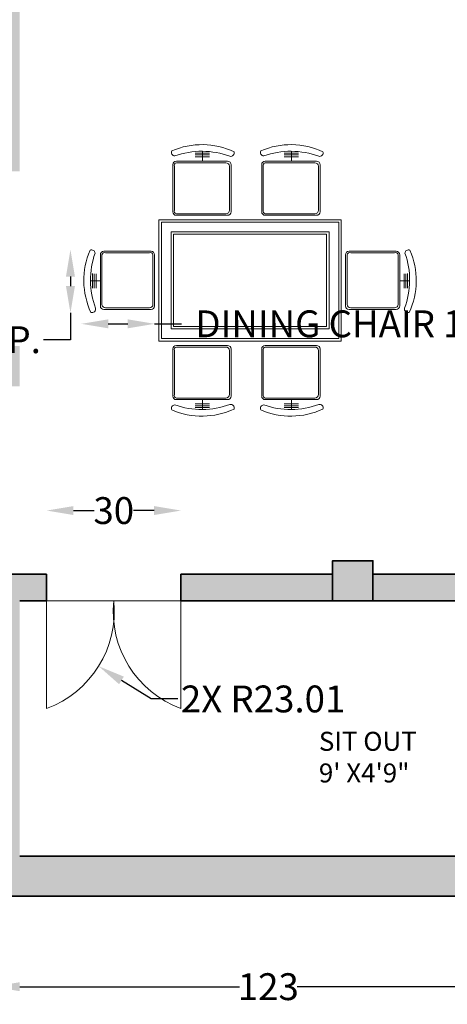
# Model space of a CAD drawing. Units: inches. Extents: x 1994 to 3075, y 3517 to 3950.
# Tile 53 of 58: x 2816 to 2912, y 3517 to 3737. Entities that reach past the tile are written whole.
import ezdxf

# ---------------------------------------------------------------- set-up
doc = ezdxf.new("R2010")
doc.units = ezdxf.units.IN
for name, color, linetype, lineweight in [('A-ANNO-DIMS', 2, 'Continuous', 18), ('A-AREA-IDEN', 7, 'Continuous', 18), ('A-COLS', 7, 'Continuous', 35), ('A-COLS-PATT', 6, 'Continuous', 13), ('A-DOOR', 3, 'Continuous', 18), ('A-FURN', 8, 'Continuous', 18), ('A-WALL', 7, 'Continuous', 35), ('A-WALL-PATT', 252, 'Continuous', 13)]:
    doc.layers.add(name, color=color, linetype=linetype, lineweight=lineweight)
doc.styles.get("Standard").update_dxf_attribs({"font": 'arial.ttf'})
doc.dimstyles.get("Standard").update_dxf_attribs({"dimtxt": 6, "dimasz": 6, "dimexe": 0.18, "dimexo": 0.0625, "dimgap": 0.09, "dimtad": 0, "dimtih": 1, "dimtoh": 1, "dimdec": 4, "dimzin": 0, "dimdsep": 46, "dimlunit": 4, "dimtxsty": 'Standard', "dimcen": 0.09, "dimse1": 1, "dimse2": 1, "dimadec": 0, "dimazin": 0, "dimtfac": 1, "dimtdec": 4, "dimtofl": 0, "dimtmove": 0, "dimatfit": 3, "dimfxl": 1, "dimtolj": 1, "dimtzin": 0, "dimarcsym": 0})

# ---------------------------------------------------------------- blocks, each defined once
blk = doc.blocks.new('CHAIR-DINING')
for p, q in [((12.53, 15.8), (1.1, 15.8)), ((12.17, 15.44), (1.1, 15.44)), ((0.3, 15), (0.3, 4.49)), ((0.66, 14.64), (0.66, 4.85)), ((12.97, 4.85), (12.97, 14.64)), ((13.33, 4.49), (13.33, 15)), ((1.1, 4.05), (12.17, 4.05)), ((1.1, 3.69), (12.53, 3.69)), ((5.32, 2.73), (8.52, 2.73)), ((5.32, 2.3), (8.52, 2.3)), ((6.92, 3.69), (6.92, 1.56)), ((5.29, 1.93), (8.52, 1.93))]:
    blk.add_line(p, q)
for centre, radius, start, end in [((1.1, 15), 0.8, 90, 180), ((1.17, 14.88), 0.564, 96.7142, 205.1766), ((12.17, 14.64), 0.8, 0, 90), ((12.53, 15), 0.8, 0, 90), ((1.1, 4.49), 0.8, 180, 270), ((1.17, 4.61), 0.564, 154.8234, 263.2858), ((12.17, 4.85), 0.8, 270, 0), ((12.53, 4.49), 0.8, 270, 0), ((0.77, 1.75), 0.766, 91.9354, 207.5327), ((6.77, 19.53), 18.05, 250.4914, 290.3763), ((13.22, 1.83), 0.8, 342.1953, 102.3742), ((6.83, 16.94), 16.94, 246.5531, 294.9844)]:
    blk.add_arc(centre, radius, start, end)
blk = doc.blocks.new('*D15')
at = {"layer": 'A-ANNO-DIMS', "color": 0, "lineweight": -2, "transparency": 16777216}
for p, q in [((2835.85, 3669.06), (2840.19, 3669.06)), ((2846.19, 3669.06), (2852.19, 3669.06))]:
    blk.add_line(p, q, dxfattribs=at)
at = {"layer": 'A-ANNO-DIMS', "color": 0, "transparency": 16777216}
for points in [[(2835.85, 3670.06), (2835.85, 3668.06), (2829.85, 3669.06)], [(2840.19, 3670.06), (2840.19, 3668.06), (2846.19, 3669.06)]]:
    blk.add_solid(points, dxfattribs=at)
at = {"layer": 'Defpoints', "color": 0, "transparency": 16777216}
for p in [(2829.85, 3671.51), (2846.19, 3671.51), (2846.19, 3669.06)]:
    blk.add_point(p, dxfattribs=at)
at = {"layer": 'A-ANNO-DIMS', "color": 0, "transparency": 16777216, "insert": (2896.77, 3669.06), "char_height": 6, "attachment_point": 5}
blk.add_mtext('\\A1;DINING CHAIR 16 TYP.', dxfattribs=at)
blk = doc.blocks.new('*D16')
at = {"layer": 'A-ANNO-DIMS', "color": 0, "lineweight": -2, "transparency": 16777216}
for p, q in [((2827.4, 3679.62), (2827.4, 3677.51)), ((2827.4, 3671.51), (2827.4, 3665.51)), ((2827.4, 3665.51), (2821.4, 3665.51))]:
    blk.add_line(p, q, dxfattribs=at)
at = {"layer": 'A-ANNO-DIMS', "color": 0, "transparency": 16777216}
for points in [[(2826.4, 3679.62), (2828.4, 3679.62), (2827.4, 3685.62)], [(2826.4, 3677.51), (2828.4, 3677.51), (2827.4, 3671.51)]]:
    blk.add_solid(points, dxfattribs=at)
at = {"layer": 'Defpoints', "color": 0, "transparency": 16777216}
for p in [(2829.85, 3685.62), (2827.4, 3671.51), (2829.85, 3671.51)]:
    blk.add_point(p, dxfattribs=at)
at = {"layer": 'A-ANNO-DIMS', "color": 0, "transparency": 16777216, "insert": (2806.99, 3665.51), "char_height": 6, "attachment_point": 5}
blk.add_mtext('\\A1;14 TYP.', dxfattribs=at)
blk = doc.blocks.new('*D34')
at = {"layer": 'A-ANNO-DIMS', "color": 0, "lineweight": -2, "transparency": 16777216}
for p, q in [((2816.07, 3520.93), (2865.14, 3520.93)), ((2927.07, 3520.93), (2878.01, 3520.93))]:
    blk.add_line(p, q, dxfattribs=at)
at = {"layer": 'A-ANNO-DIMS', "color": 0, "transparency": 16777216}
for points in [[(2816.07, 3521.93), (2816.07, 3519.93), (2810.07, 3520.93)], [(2927.07, 3521.93), (2927.07, 3519.93), (2933.07, 3520.93)]]:
    blk.add_solid(points, dxfattribs=at)
at = {"layer": 'Defpoints', "color": 0, "transparency": 16777216}
for p in [(2810.07, 3541.13), (2933.07, 3541.13), (2933.07, 3520.93)]:
    blk.add_point(p, dxfattribs=at)
at = {"layer": 'A-ANNO-DIMS', "color": 0, "transparency": 16777216, "insert": (2871.57, 3520.93), "char_height": 6, "attachment_point": 5}
blk.add_mtext('\\A1;123', dxfattribs=at)
blk = doc.blocks.new('*D49')
at = {"layer": 'A-ANNO-DIMS', "color": 0, "lineweight": -2, "transparency": 16777216}
for p, q in [((2828.07, 3627.33), (2832.7, 3627.33)), ((2846.07, 3627.33), (2841.45, 3627.33))]:
    blk.add_line(p, q, dxfattribs=at)
at = {"layer": 'A-ANNO-DIMS', "color": 0, "transparency": 16777216}
for points in [[(2828.07, 3628.33), (2828.07, 3626.33), (2822.07, 3627.33)], [(2846.07, 3628.33), (2846.07, 3626.33), (2852.07, 3627.33)]]:
    blk.add_solid(points, dxfattribs=at)
at = {"layer": 'Defpoints', "color": 0, "transparency": 16777216}
for p in [(2852.07, 3627.33), (2822.07, 3607.13), (2852.07, 3607.13)]:
    blk.add_point(p, dxfattribs=at)
at = {"layer": 'A-ANNO-DIMS', "color": 0, "transparency": 16777216, "insert": (2837.07, 3627.33), "char_height": 6, "attachment_point": 5}
blk.add_mtext('\\A1;30', dxfattribs=at)
blk = doc.blocks.new('*D56')
at = {"layer": 'A-ANNO-DIMS', "color": 0, "lineweight": -2, "transparency": 16777216}
for p, q in [((2814.1, 3604.74), (2814.28, 3604.74)), ((2814.19, 3604.65), (2814.19, 3604.83)), ((2845.41, 3585.23), (2838.79, 3589.37)), ((2851.41, 3585.23), (2845.41, 3585.23))]:
    blk.add_line(p, q, dxfattribs=at)
at = {"layer": 'A-ANNO-DIMS', "color": 0, "transparency": 16777216}
blk.add_solid([(2839.32, 3590.22), (2838.26, 3588.52), (2833.7, 3592.55)], dxfattribs=at)
at = {"layer": 'Defpoints', "color": 0, "transparency": 16777216}
for p in [(2814.19, 3604.74), (2833.7, 3592.55)]:
    blk.add_point(p, dxfattribs=at)
at = {"layer": 'A-ANNO-DIMS', "color": 0, "transparency": 16777216, "insert": (2870.41, 3585.23), "char_height": 6, "attachment_point": 5}
blk.add_mtext('\\A1;2X R23.01', dxfattribs=at)

msp = doc.modelspace()

# ---------------------------------------------------------------- hatches: boundary and pattern name
at = {"layer": 'A-COLS-PATT'}
h = msp.add_hatch(color=256, dxfattribs=at)
h.dxf.hatch_style = 1
h.paths.add_polyline_path([(2678.072, 3914.1269), (2669.072, 3914.1269), (2669.072, 3905.1269), (2678.072, 3905.1269)])
h.paths.add_polyline_path([(2816.072, 3914.1269), (2807.072, 3914.1269), (2807.072, 3905.1269), (2816.072, 3905.1269)])
h.paths.add_polyline_path([(2894.9096, 3914.1269), (2885.9096, 3914.1269), (2885.9096, 3905.1269), (2894.9096, 3905.1269)])
h.paths.add_polyline_path([(3033.072, 3914.1269), (3024.072, 3914.1269), (3024.072, 3905.1269), (3033.072, 3905.1269)])
h.paths.add_polyline_path([(3033.072, 3764.1269), (3024.072, 3764.1269), (3024.072, 3755.1269), (3033.072, 3755.1269)])
h.paths.add_polyline_path([(2895.072, 3764.1269), (2886.072, 3764.1269), (2886.072, 3755.1269), (2895.072, 3755.1269)])
h.paths.add_polyline_path([(2816.072, 3764.1269), (2807.072, 3764.1269), (2807.072, 3755.1269), (2816.072, 3755.1269)])
h.paths.add_polyline_path([(2678.072, 3764.1269), (2669.072, 3764.1269), (2669.072, 3755.1269), (2678.072, 3755.1269)])
h.paths.add_polyline_path([(2678.072, 3664.1269), (2669.072, 3664.1269), (2669.072, 3655.1269), (2678.072, 3655.1269)])
h.paths.add_polyline_path([(2816.072, 3664.1269), (2807.072, 3664.1269), (2807.072, 3655.1269), (2816.072, 3655.1269)])
h.paths.add_polyline_path([(3033.072, 3616.1269), (3024.072, 3616.1269), (3024.072, 3607.1269), (3033.072, 3607.1269)])
h.paths.add_polyline_path([(2894.9096, 3616.1269), (2885.9096, 3616.1269), (2885.9096, 3607.1269), (2894.9096, 3607.1269)])
h.paths.add_polyline_path([(2816.072, 3559.1269), (2807.072, 3559.1269), (2807.072, 3550.1269), (2816.072, 3550.1269)])
h.paths.add_polyline_path([(2678.072, 3559.1269), (2669.072, 3559.1269), (2669.072, 3550.1269), (2678.072, 3550.1269)])
at = {"layer": 'A-WALL-PATT'}
h = msp.add_hatch(color=256, dxfattribs=at)
h.dxf.hatch_style = 1
h.paths.add_polyline_path([(2678.072, 3755.1269), (2669.072, 3755.1269), (2669.072, 3718.5523), (2678.072, 3718.5523)])
h.paths.add_polyline_path([(2807.072, 3761.1269), (2678.072, 3761.1269), (2678.072, 3755.1269), (2807.072, 3755.1269)])
h.paths.add_polyline_path([(2678.072, 3812.7371), (2669.072, 3812.7371), (2669.072, 3809.7371), (2669.072, 3764.1269), (2678.072, 3764.1269)])
h.paths.add_polyline_path([(2678.072, 3905.1269), (2669.072, 3905.1269), (2669.072, 3868.7491), (2678.072, 3868.7491)])
h.paths.add_polyline_path([(2723.826, 3914.1269), (2720.826, 3914.1269), (2678.072, 3914.1269), (2678.072, 3905.1269), (2723.826, 3905.1269)])
h.paths.add_polyline_path([(2807.072, 3914.1269), (2779.838, 3914.1269), (2779.838, 3905.1269), (2807.072, 3905.1269)])
h.paths.add_polyline_path([(2837.6979, 3914.1269), (2834.6979, 3914.1269), (2820.9062, 3914.1269), (2816.072, 3914.1269), (2816.072, 3905.1269), (2837.6979, 3905.1269)])
h.paths.add_polyline_path([(2885.9096, 3914.1269), (2869.71, 3914.1269), (2869.71, 3905.1269), (2876.9183, 3905.1269), (2885.9096, 3905.1269)])
h.paths.add_polyline_path([(2933.6904, 3914.1269), (2930.6904, 3914.1269), (2894.9096, 3914.1269), (2894.9096, 3905.1269), (2933.6904, 3905.1269)])
h.paths.add_polyline_path([(3024.072, 3914.1269), (2989.7025, 3914.1269), (2989.7025, 3905.1269), (3024.072, 3905.1269)])
h.paths.add_polyline_path([(3033.072, 3905.1269), (3024.072, 3905.1269), (3024.072, 3861.4192), (3033.072, 3861.4192)])
h.paths.add_polyline_path([(3033.072, 3805.4072), (3024.072, 3805.4072), (3024.072, 3764.1269), (3033.072, 3764.1269)])
h.paths.add_polyline_path([(3033.072, 3755.1269), (3024.072, 3755.1269), (3024.072, 3732.1247), (3033.072, 3732.1247), (3033.072, 3735.1247)])
h.paths.add_polyline_path([(3024.072, 3761.1269), (2895.072, 3761.1269), (2895.072, 3755.1269), (3024.072, 3755.1269)])
h.paths.add_polyline_path([(3033.072, 3676.1126), (3024.072, 3676.1126), (3024.072, 3616.1269), (3033.072, 3616.1269)])
h.paths.add_polyline_path([(3024.072, 3613.1269), (2959.4908, 3613.1269), (2959.4908, 3607.1269), (3024.072, 3607.1269)])
h.paths.add_polyline_path([(2914.1254, 3613.1269), (2894.9096, 3613.1269), (2894.9096, 3607.1269), (2914.1254, 3607.1269)])
h.paths.add_polyline_path([(2885.9096, 3613.1269), (2852.072, 3613.1269), (2852.072, 3607.1269), (2885.9096, 3607.1269)])
h.paths.add_polyline_path([(2822.072, 3613.1269), (2810.072, 3613.1269), (2810.072, 3559.1269), (2816.072, 3559.1269), (2816.072, 3607.1269), (2822.072, 3607.1269)])
h.paths.add_polyline_path([(2933.072, 3607.1269), (2924.072, 3607.1269), (2924.072, 3550.1269), (2892.072, 3550.1269), (2816.072, 3550.1269), (2810.072, 3550.1269), (2810.072, 3541.1269), (2892.072, 3541.1269), (2933.072, 3541.1269)])
h.paths.add_polyline_path([(2807.072, 3559.1269), (2678.072, 3559.1269), (2678.072, 3550.1269), (2807.072, 3550.1269)])
h.paths.add_polyline_path([(2678.072, 3655.1269), (2669.072, 3655.1269), (2669.072, 3559.1269), (2678.072, 3559.1269)])
h.paths.add_polyline_path([(2678.072, 3686.5403), (2669.072, 3686.5403), (2669.072, 3664.1269), (2678.072, 3664.1269)])
h.paths.add_polyline_path([(2807.072, 3661.1269), (2678.072, 3661.1269), (2678.072, 3655.1269), (2807.072, 3655.1269)])
h.paths.add_polyline_path([(2816.072, 3755.1269), (2810.072, 3755.1269), (2810.072, 3703.1269), (2816.072, 3703.1269)])
h.paths.add_polyline_path([(2816.072, 3905.1269), (2810.072, 3905.1269), (2810.072, 3803.1269), (2816.072, 3803.1269), (2816.072, 3815.1269)])
h.paths.add_polyline_path([(2886.072, 3821.1269), (2852.072, 3821.1269), (2852.072, 3815.1269), (2886.072, 3815.1269)])
h.paths.add_polyline_path([(2822.072, 3821.1269), (2816.072, 3821.1269), (2816.072, 3815.1269), (2822.072, 3815.1269)])
h.paths.add_polyline_path([(2892.072, 3905.1269), (2886.072, 3905.1269), (2886.072, 3803.1269), (2892.072, 3803.1269)])

# ---------------------------------------------------------------- linework, layer by layer
at = {"layer": 'A-COLS'}
msp.add_lwpolyline([(2885.9096, 3607.1269), (2894.9096, 3607.1269), (2894.9096, 3616.1269), (2885.9096, 3616.1269)], close=True, dxfattribs=at)
at = {"layer": 'A-DOOR'}
for p, q in [((2822.072, 3607.1269), (2852.072, 3607.1269)), ((2822.072, 3607.1269), (2822.072, 3583.1269)), ((2852.072, 3607.1269), (2852.072, 3583.1269))]:
    msp.add_line(p, q, dxfattribs=at)
for centre, start, end in [((2814.1856, 3604.7434), 290.043695, 5.945539), ((2859.9585, 3604.7434), 174.054461, 249.956305)]:
    msp.add_arc(centre, 23.0102, start, end, dxfattribs=at)
at = {"layer": 'A-FURN'}
for p, q in [((2847.1497, 3665.2084), (2847.1497, 3692.3322)), ((2847.1497, 3692.3322), (2887.8354, 3692.3322)), ((2887.8354, 3692.3322), (2887.8354, 3665.2084)), ((2847.6922, 3665.7509), (2847.6922, 3691.7897)), ((2847.6922, 3691.7897), (2887.2929, 3691.7897)), ((2887.2929, 3691.7897), (2887.2929, 3665.7509)), ((2849.8621, 3667.9208), (2849.8621, 3689.6198)), ((2849.8621, 3689.6198), (2885.123, 3689.6198)), ((2850.4046, 3668.4632), (2850.4046, 3689.0773)), ((2850.4046, 3689.0773), (2884.5806, 3689.0773)), ((2884.5806, 3689.0773), (2884.5806, 3668.4632)), ((2885.123, 3689.6198), (2885.123, 3667.9208)), ((2884.5806, 3668.4632), (2850.4046, 3668.4632)), ((2885.123, 3667.9208), (2849.8621, 3667.9208)), ((2887.8354, 3665.2084), (2847.1497, 3665.2084)), ((2887.2929, 3665.7509), (2847.6922, 3665.7509))]:
    msp.add_line(p, q, dxfattribs=at)
at = {"layer": 'A-WALL'}
for p, q in [((2810.072, 3613.1269), (2822.072, 3613.1269)), ((2822.072, 3613.1269), (2822.072, 3607.1269)), ((2852.072, 3607.1269), (2852.072, 3613.1269)), ((2852.072, 3613.1269), (2885.9096, 3613.1269)), ((2894.9096, 3613.1269), (3024.072, 3613.1269)), ((2822.072, 3607.1269), (2816.072, 3607.1269)), ((2886.072, 3607.1269), (2852.072, 3607.1269)), ((2892.072, 3607.1269), (2886.072, 3607.1269)), ((2892.072, 3607.1269), (2924.072, 3607.1269)), ((2892.072, 3550.1269), (2816.072, 3550.1269)), ((2892.072, 3550.1269), (2924.072, 3550.1269)), ((2892.072, 3541.1269), (2810.072, 3541.1269)), ((2892.072, 3541.1269), (2933.072, 3541.1269))]:
    msp.add_line(p, q, dxfattribs=at)

# ---------------------------------------------------------------- block references
at = {"layer": 'A-FURN', "extrusion": (0, 0, -1), "zscale": -1}
for p, rotation in [((-2849.941, 3709.1086), 180), ((-2869.7964, 3709.1086), 180), ((-2904.5999, 3685.5852), 269.9999999961732)]:
    msp.add_blockref('CHAIR-DINING', p, dxfattribs=dict(at, rotation=rotation))
at = {"layer": 'A-FURN', "rotation": 269.9999999960863}
msp.add_blockref('CHAIR-DINING', (2830.3853, 3685.5852), dxfattribs=at)
at = {"layer": 'A-FURN'}
for p in [(2849.941, 3648.432), (2869.7964, 3648.432)]:
    msp.add_blockref('CHAIR-DINING', p, dxfattribs=at)

# ---------------------------------------------------------------- texts
at = {"layer": 'A-AREA-IDEN', "insert": (2882.8634, 3577.8877), "char_height": 4.24528, "attachment_point": 1}
msp.add_mtext_dynamic_manual_height_columns('SIT OUT\\P9\' X4\'9"', width=102.693633, gutter_width=21.2264, heights=[0], dxfattribs=at)

# ---------------------------------------------------------------- dimensions: what is measured, and where the dimension line sits
at = {"layer": 'A-ANNO-DIMS'}
for base, p1, p2, angle, text, picture, middle in [((2846.1884, 3669.062), (2829.8543, 3671.5122), (2846.1884, 3671.5122), 360, 'DINING CHAIR <> TYP.', '*D15', (2896.7689, 3669.062)), ((2827.4041, 3671.5122), (2829.8543, 3685.6199), (2829.8543, 3671.5122), 270, '<> TYP.', '*D16', (2806.9935, 3665.5122))]:
    dim = msp.add_linear_dim(base=base, p1=p1, p2=p2, angle=angle, text=text, dimstyle='Standard', override={"dimdec": 0, "dimlfac": 1, "dimrnd": 0, "dimzin": 0, "dimdsep": 46, "dimlunit": 2}, dxfattribs=at)
    dim.commit()
    dim.dimension.update_dxf_attribs({"geometry": picture, "text_midpoint": middle})
for base, p1, p2, picture, middle in [((2852.072, 3627.3269), (2822.072, 3607.1269), (2852.072, 3607.1269), '*D49', (2837.072, 3627.3269)), ((2933.072, 3520.9269), (2810.072, 3541.1269), (2933.072, 3541.1269), '*D34', (2871.572, 3520.9269))]:
    dim = msp.add_linear_dim(base=base, p1=p1, p2=p2, dimstyle='Standard', override={"dimdec": 0, "dimlfac": 1, "dimrnd": 0, "dimzin": 0, "dimdsep": 46, "dimlunit": 2}, dxfattribs=at)
    dim.commit()
    dim.dimension.update_dxf_attribs({"geometry": picture, "text_midpoint": middle})
dim = msp.add_radius_dim(center=(2814.1856, 3604.7434), mpoint=(2833.6982, 3592.5479), text='2X <>', dimstyle='Standard', override={"dimdec": 2, "dimlfac": 1, "dimrnd": 0, "dimzin": 0, "dimdsep": 46, "dimlunit": 2}, dxfattribs=at)
dim.commit()
dim.dimension.update_dxf_attribs({"geometry": '*D56', "text_midpoint": (2870.4084, 3585.2306), "dimtype": 164})

doc.saveas('drawing.dxf')
